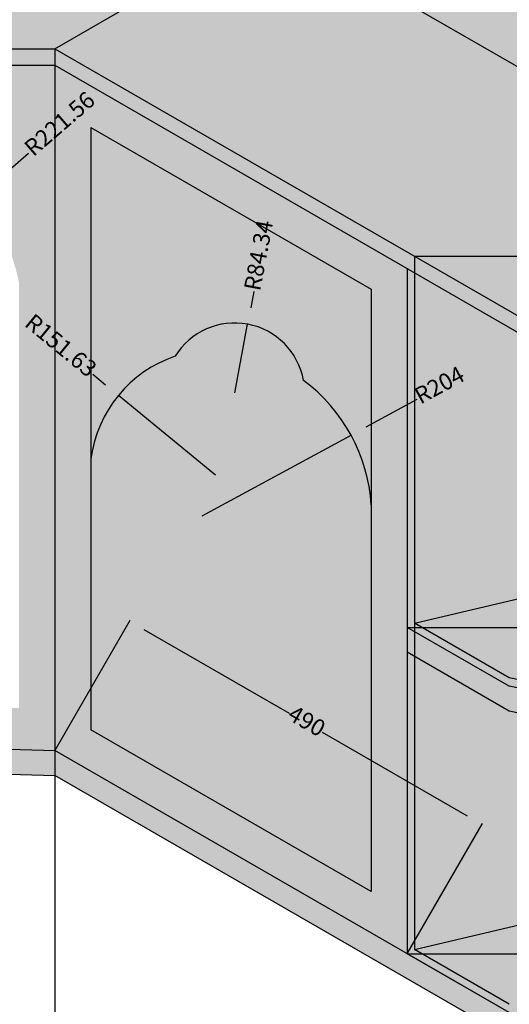
# Model space of a CAD drawing. Units: millimetres. Extents: x 78378 to 86415, y 148682 to 152721.
# Tile 10 of 18: x 80650 to 81240, y 149308 to 150495. Entities that reach past the tile are written whole.
import ezdxf

# ---------------------------------------------------------------- set-up
doc = ezdxf.new("R2010")
doc.units = ezdxf.units.MM
for name, color, linetype, lineweight in [('A-ANNO-DIMS', 2, 'Continuous', 18), ('A-FURN', 4, 'Continuous', 25), ('A-FURN-PATT', 32, 'Continuous', 13)]:
    doc.layers.add(name, color=color, linetype=linetype, lineweight=lineweight)
doc.styles.get("Standard").update_dxf_attribs({"font": 'arial.ttf'})
doc.dimstyles.new('ISO-25', dxfattribs={"dimtxt": 20, "dimasz": 20, "dimexe": 1.25, "dimexo": 0.625, "dimtad": 0, "dimdec": 1, "dimtxsty": 'Standard', "dimcen": 2.5, "dimadec": 0, "dimazin": 0, "dimtfac": 1, "dimtdec": 1, "dimtmove": 0, "dimatfit": 3, "dimfxl": 1, "dimarcsym": 0})

# ---------------------------------------------------------------- blocks, each defined once
blk = doc.blocks.new('*D27')
at = {"layer": 'A-ANNO-DIMS', "color": 0, "lineweight": -2, "transparency": 16777216}
for p, q in [((80692.9, 149614.5), (80783.2, 149771)), ((80799.9, 149759.9), (80974.8, 149658.9)), ((81189.7, 149534.9), (81014.8, 149635.8)), ((81117.3, 149369.5), (81207.6, 149526))]:
    blk.add_line(p, q, dxfattribs=at)
at = {"layer": 'A-ANNO-DIMS', "color": 0, "transparency": 16777216}
for points in [[(80801.6, 149762.8), (80798.3, 149757), (80782.6, 149769.9)], [(81191.3, 149537.8), (81188, 149532), (81207, 149524.9)]]:
    blk.add_solid(points, dxfattribs=at)
at = {"layer": 'Defpoints', "color": 0, "transparency": 16777216}
for p in [(80692.6, 149614), (81207, 149524.9), (81117, 149369)]:
    blk.add_point(p, dxfattribs=at)
at = {"layer": 'A-ANNO-DIMS', "color": 0, "transparency": 16777216, "insert": (80994.8, 149647.4), "char_height": 20, "attachment_point": 5, "rotation": 330}
blk.add_mtext('490', dxfattribs=at)
blk = doc.blocks.new('*D28')
at = {"layer": 'A-ANNO-DIMS', "color": 0, "lineweight": -2, "transparency": 16777216}
for p, q in [((81117.6, 149762.4), (81956.4, 149762.4)), ((81955.2, 149742.4), (81955.2, 149600)), ((81955.2, 149389), (81955.2, 149531.4)), ((81117.6, 149369), (81956.4, 149369))]:
    blk.add_line(p, q, dxfattribs=at)
at = {"layer": 'A-ANNO-DIMS', "color": 0, "transparency": 16777216}
for points in [[(81951.8, 149742.4), (81958.5, 149742.4), (81955.2, 149762.4)], [(81951.8, 149389), (81958.5, 149389), (81955.2, 149369)]]:
    blk.add_solid(points, dxfattribs=at)
at = {"layer": 'Defpoints', "color": 0, "transparency": 16777216}
for p in [(81117, 149762.4), (81955.2, 149762.4), (81117, 149369)]:
    blk.add_point(p, dxfattribs=at)
at = {"layer": 'A-ANNO-DIMS', "color": 0, "transparency": 16777216, "insert": (81955.2, 149565.7), "char_height": 20, "attachment_point": 5, "rotation": 90}
blk.add_mtext('393.4', dxfattribs=at)
blk = doc.blocks.new('*D29')
at = {"layer": 'A-ANNO-DIMS', "color": 0, "lineweight": -2, "transparency": 16777216}
for p, q in [((81126.3, 150210), (81956.4, 150210)), ((81955.2, 150190), (81955.2, 150021)), ((81955.2, 149782.4), (81955.2, 149951.4)), ((81117.6, 149762.4), (81956.4, 149762.4))]:
    blk.add_line(p, q, dxfattribs=at)
at = {"layer": 'A-ANNO-DIMS', "color": 0, "transparency": 16777216}
for points in [[(81951.8, 150190), (81958.5, 150190), (81955.2, 150210)], [(81951.8, 149782.4), (81958.5, 149782.4), (81955.2, 149762.4)]]:
    blk.add_solid(points, dxfattribs=at)
at = {"layer": 'Defpoints', "color": 0, "transparency": 16777216}
for p in [(81125.6, 150210), (81955.2, 150210), (81117, 149762.4)]:
    blk.add_point(p, dxfattribs=at)
at = {"layer": 'A-ANNO-DIMS', "color": 0, "transparency": 16777216, "insert": (81955.2, 149986.2), "char_height": 20, "attachment_point": 5, "rotation": 90}
blk.add_mtext('447.6', dxfattribs=at)
blk = doc.blocks.new('*D32')
at = {"layer": 'A-ANNO-DIMS', "color": 0, "lineweight": -2, "transparency": 16777216}
for p, q in [((80086.4, 150459.4), (80086.4, 148693.8)), ((80692.6, 150459.4), (80692.6, 148693.8)), ((80106.4, 148695), (80355.2, 148695)), ((80672.6, 148695), (80423.8, 148695))]:
    blk.add_line(p, q, dxfattribs=at)
at = {"layer": 'A-ANNO-DIMS', "color": 0, "transparency": 16777216}
for points in [[(80106.4, 148698.3), (80106.4, 148691.7), (80086.4, 148695)], [(80672.6, 148698.3), (80672.6, 148691.7), (80692.6, 148695)]]:
    blk.add_solid(points, dxfattribs=at)
at = {"layer": 'Defpoints', "color": 0, "transparency": 16777216}
for p in [(80086.4, 150460), (80692.6, 150460), (80692.6, 148695)]:
    blk.add_point(p, dxfattribs=at)
at = {"layer": 'A-ANNO-DIMS', "color": 0, "transparency": 16777216, "insert": (80389.5, 148695), "char_height": 20, "attachment_point": 5}
blk.add_mtext('606.2', dxfattribs=at)
blk = doc.blocks.new('*D64')
at = {"layer": 'A-ANNO-DIMS', "color": 0, "lineweight": -2, "transparency": 16777216}
for p, q in [((80660.8, 150333.8), (80614.5, 150293.7)), ((80431.9, 150135.6), (80599.4, 150280.6))]:
    blk.add_line(p, q, dxfattribs=at)
at = {"layer": 'A-ANNO-DIMS', "color": 0, "transparency": 16777216}
blk.add_solid([(80612.3, 150296.2), (80616.7, 150291.2), (80599.4, 150280.6)], dxfattribs=at)
at = {"layer": 'Defpoints', "color": 0, "transparency": 16777216}
for p in [(80599.4, 150280.6), (80431.9, 150135.6)]:
    blk.add_point(p, dxfattribs=at)
at = {"layer": 'A-ANNO-DIMS', "color": 0, "transparency": 16777216, "insert": (80699.9, 150367.7), "char_height": 20, "attachment_point": 5, "rotation": 40.8938}
blk.add_mtext('R221.56', dxfattribs=at)
blk = doc.blocks.new('*D66')
at = {"layer": 'A-ANNO-DIMS', "color": 0, "lineweight": -2, "transparency": 16777216}
for p, q in [((81128.6, 150037.1), (81067, 150003.6)), ((80870.1, 149896.7), (81049.4, 149994))]:
    blk.add_line(p, q, dxfattribs=at)
at = {"layer": 'A-ANNO-DIMS', "color": 0, "transparency": 16777216}
blk.add_solid([(81065.4, 150006.5), (81068.6, 150000.7), (81049.4, 149994)], dxfattribs=at)
at = {"layer": 'Defpoints', "color": 0, "transparency": 16777216}
for p in [(81049.4, 149994), (80870.1, 149896.7)]:
    blk.add_point(p, dxfattribs=at)
at = {"layer": 'A-ANNO-DIMS', "color": 0, "transparency": 16777216, "insert": (81157, 150052.4), "char_height": 20, "attachment_point": 5, "rotation": 28.4955}
blk.add_mtext('R204', dxfattribs=at)
blk = doc.blocks.new('*D67')
at = {"layer": 'A-ANNO-DIMS', "color": 0, "lineweight": -2, "transparency": 16777216}
for p, q in [((80738.3, 150067.6), (80753.7, 150054.9)), ((80886.2, 149945.8), (80769.1, 150042.1))]:
    blk.add_line(p, q, dxfattribs=at)
at = {"layer": 'A-ANNO-DIMS', "color": 0, "transparency": 16777216}
blk.add_solid([(80755.8, 150057.4), (80751.6, 150052.3), (80769.1, 150042.1)], dxfattribs=at)
at = {"layer": 'Defpoints', "color": 0, "transparency": 16777216}
for p in [(80769.1, 150042.1), (80886.2, 149945.8)]:
    blk.add_point(p, dxfattribs=at)
at = {"layer": 'A-ANNO-DIMS', "color": 0, "transparency": 16777216, "insert": (80698.3, 150100.4), "char_height": 20, "attachment_point": 5, "rotation": 320.5336}
blk.add_mtext('R151.63', dxfattribs=at)
blk = doc.blocks.new('*D68')
at = {"layer": 'A-ANNO-DIMS', "color": 0, "lineweight": -2, "transparency": 16777216}
for p, q in [((80932.2, 150167.2), (80928.5, 150147.6)), ((80909.2, 150045), (80924.8, 150127.9))]:
    blk.add_line(p, q, dxfattribs=at)
at = {"layer": 'A-ANNO-DIMS', "color": 0, "transparency": 16777216}
blk.add_solid([(80925.3, 150148.2), (80931.8, 150147), (80924.8, 150127.9)], dxfattribs=at)
at = {"layer": 'Defpoints', "color": 0, "transparency": 16777216}
for p in [(80924.8, 150127.9), (80909.2, 150045)]:
    blk.add_point(p, dxfattribs=at)
at = {"layer": 'A-ANNO-DIMS', "color": 0, "transparency": 16777216, "insert": (80940.4, 150210.4), "char_height": 20, "attachment_point": 5, "rotation": 79.3222}
blk.add_mtext('R84.34', dxfattribs=at)

msp = doc.modelspace()

# ---------------------------------------------------------------- hatches: boundary and pattern name
at = {"layer": 'A-FURN-PATT'}
h = msp.add_hatch(color=256, dxfattribs=at)
h.dxf.hatch_style = 1
h.paths.add_polyline_path([(78839.3276, 151040.0076), (78579.52, 151190.0076), (78579.52, 150470.0076), (78839.3276, 150320.0076)])
h.paths.add_polyline_path([(79073.1545, 150899.6469, 0.277779695), (79002.2645, 150996.3205, 0.791083931), (78917.9567, 150978.8719, 0.180448316), (78856.6481, 150853.0138), (78856.6481, 150350.6973), (79073.1545, 150484.318)])
h.paths.add_polyline_path([(79073.1545, 151175.0076), (78856.6481, 151050.0076), (78856.6481, 150853.0138, -0.180448316), (78917.9567, 150978.8719, -0.791083931), (79002.2645, 150996.3205, -0.277779695), (79073.1545, 150899.6469)])
h.paths.add_polyline_path([(79341.6224, 151350.0076), (79099.1352, 151490.0076), (78596.8405, 151200.0076), (78839.3276, 151060.0076)])
h.paths.add_polyline_path([(79904.5389, 151675.0076), (79662.0518, 151815.0076), (79099.1352, 151490.0076), (79341.6224, 151350.0076)])
h.paths.add_polyline_path([(80389.5131, 151955.0076), (80389.5131, 152235.0076), (79662.0518, 151815.0076), (79904.5389, 151675.0076)])
h.paths.add_polyline_path([(80389.5131, 151955.0076), (80164.3465, 151825.0076), (80164.3465, 151105.0076), (80614.6797, 151105.0076), (80614.6797, 151825.0076)])
edge = h.paths.add_edge_path(flags=16)
edge.add_spline(control_points=[(80216.308, 151728.251), (80227.1854, 151732.981), (80256.3301, 151745.6544), (80298.41, 151761.9595), (80340.2597, 151805.855), (80391.0771, 151782.0404), (80454.0396, 151805.7581), (80496.5007, 151742.4095), (80543.8218, 151733.4043), (80562.7182, 151729.8083)], knot_values=[0, 0, 0, 0, 35.543746761, 95.235753469, 136.367675126, 200.932981967, 236.726410811, 322.889934976, 380.170273667, 380.170273667, 380.170273667, 380.170273667], degree=3, periodic=0)
edge.add_line((80562.7182, 151729.8083), (80562.7182, 151165.0076))
edge.add_line((80562.7182, 151165.0076), (80216.308, 151165.0076))
edge.add_line((80216.308, 151165.0076), (80216.308, 151728.251))
h.paths.add_polyline_path([(80632.0002, 152095.0076), (80389.5131, 152235.0076), (80389.5131, 151955.0076), (80614.6797, 151825.0076), (80632.0002, 151815.0076)])
h.paths.add_polyline_path([(80867.7794, 151958.8805), (80632.0002, 152095.0076), (80632.0002, 151815.0076), (80632.0002, 151510.0076), (80867.7794, 151373.8805)])
h.paths.add_polyline_path([(80147.026, 151495.8203, 0.18918979), (80063.5671, 151597.7244, 0.788261355), (79979.2691, 151580.5832, 0.160726132), (79904.5389, 151413.5769), (79904.5389, 150955.0076), (80147.026, 151095.0076)])
h.paths.add_polyline_path([(80147.026, 151815.0076), (79904.5389, 151675.0076), (79904.5389, 151413.5769, -0.160726132), (79979.2691, 151580.5832, -0.788261355), (80063.5671, 151597.7244, -0.18918979), (80147.026, 151495.8203)])
h.paths.add_polyline_path([(79887.2184, 151645.0076), (79640.4011, 151502.5076), (79640.4011, 151262.3325, -0.160726132), (79715.1313, 151429.3387, -0.788261355), (79799.4294, 151446.48, -0.21290578), (79887.2184, 151328.7247)])
h.paths.add_polyline_path([(79799.4294, 151446.48, 0.788261355), (79715.1313, 151429.3387, 0.160726132), (79640.4011, 151262.3325), (79640.4011, 150822.5076), (79887.2184, 150965.0076), (79887.2184, 151328.7247, 0.21290578)])
h.paths.add_polyline_path([(79605.7601, 151482.5076), (79358.9429, 151340.0076), (79358.9429, 151100.0701, -0.160726132), (79433.6731, 151267.0764, -0.788261355), (79517.9711, 151284.2176, -0.21290578), (79605.7601, 151166.4623)])
h.paths.add_polyline_path([(79605.7601, 151166.4623, 0.21290578), (79517.9711, 151284.2176, 0.788261355), (79433.6731, 151267.0764, 0.160726132), (79358.9429, 151100.0701), (79358.9429, 150742.9831), (79419.0877, 150694.7323), (79605.7601, 150802.5076)])
edge = h.paths.add_edge_path(flags=0)
edge.add_spline(control_points=[(81152.4356, 151098.7676), (81105.7208, 151145.9466), (81038.6136, 151213.7208), (80882.3866, 151214.1938), (80797.4434, 151311.2997), (80711.8686, 151340.3754), (80681.7691, 151350.6023)], knot_values=[0, 0, 0, 0, 188.233441, 270.4032752, 445.451792012, 540.428588287, 540.428588287, 540.428588287, 540.428588287], degree=3, periodic=0)
edge.add_line((80683.4538, 151350.0269), (80683.4538, 151104.8792))
edge.add_line((80683.4538, 151104.8792), (81152.4356, 150851.399))
edge.add_line((81152.4356, 150851.399), (81152.4356, 151098.7676))
edge = h.paths.add_edge_path(flags=0)
edge.add_spline(control_points=[(80912.9018, 151027.1103), (80892.3742, 151034.1027), (80860.1663, 151045.0739), (80835.5097, 151068.1214), (80826.5679, 151076.4797)], knot_values=[0, 0, 0, 0, 63.98405104, 100.391424282, 100.391424282, 100.391424282, 100.391424282], degree=3, periodic=0)
edge.add_arc((80830.0414, 151081.2992), 5.9407, 100.9277276, 234.2187381, ccw=False)
edge.add_spline(control_points=[(80828.9152, 151087.1322), (80837.857, 151078.7739), (80862.5136, 151055.7263), (80894.7215, 151044.7552), (80915.2491, 151037.7628)], knot_values=[0, 0, 0, 0, 36.407373242, 100.391424282, 100.391424282, 100.391424282, 100.391424282], degree=3, periodic=0)
edge.add_arc((80914.7882, 151032.2795), 5.5026, -107.9540399, 85.195579, ccw=False)
h.paths.add_polyline_path([(81238.218, 151110.0076), (80632.0002, 151460.0076), (80632.0002, 151105.0076), (81238.218, 150755.0076)])
edge = h.paths.add_edge_path(flags=16)
edge.add_line((81152.4356, 150851.399), (80683.4538, 151104.8792))
edge.add_line((80683.4538, 151104.8792), (80683.4538, 151350.0279))
edge.add_spline(control_points=[(80681.7691, 151350.6023), (80711.8686, 151340.3754), (80797.4434, 151311.2997), (80882.3866, 151214.1938), (81038.6136, 151213.7208), (81105.7208, 151145.9466), (81152.4356, 151098.7676)], knot_values=[0, 0, 0, 0, 94.976796275, 270.025313088, 352.195147288, 540.428588287, 540.428588287, 540.428588287, 540.428588287], degree=3, periodic=0)
edge.add_line((81152.4356, 151098.7676), (81152.4356, 150851.399))
edge = h.paths.add_edge_path(flags=0)
edge.add_spline(control_points=[(80912.9018, 151027.1103), (80892.3742, 151034.1027), (80860.1663, 151045.0739), (80835.5097, 151068.1214), (80826.5679, 151076.4797)], knot_values=[0, 0, 0, 0, 63.98405104, 100.391424282, 100.391424282, 100.391424282, 100.391424282], degree=3, periodic=0)
edge.add_arc((80830.0414, 151081.2992), 5.9407, 100.9277276, 234.2187381, ccw=False)
edge.add_spline(control_points=[(80828.9152, 151087.1322), (80837.857, 151078.7739), (80862.5136, 151055.7263), (80894.7215, 151044.7552), (80915.2491, 151037.7628)], knot_values=[0, 0, 0, 0, 36.407373242, 100.391424282, 100.391424282, 100.391424282, 100.391424282], degree=3, periodic=0)
edge.add_arc((80914.7882, 151032.2795), 5.5026, -107.7417882, 85.195579, ccw=False)
h.paths.add_polyline_path([(81498.0256, 151255.0076), (81238.218, 151110.0076), (81238.218, 150755.0076), (81498.0256, 150905.0076)])
edge = h.paths.add_edge_path(flags=16)
edge.add_spline(control_points=[(81152.4356, 151098.7676), (81105.7208, 151145.9466), (81038.6136, 151213.7208), (80882.3866, 151214.1938), (80797.4434, 151311.2997), (80711.8686, 151340.3754), (80681.7691, 151350.6023)], knot_values=[0, 0, 0, 0, 188.233441, 270.4032752, 445.451792012, 540.428588287, 540.428588287, 540.428588287, 540.428588287], degree=3, periodic=0)
edge.add_line((80683.4538, 151350.0279), (80683.4538, 151104.8792))
edge.add_line((80683.4538, 151104.8792), (81152.4356, 150851.399))
edge.add_line((81152.4356, 150851.399), (81152.4356, 151098.7676))
h.paths.add_polyline_path([(81453.9904, 151280.4314), (80867.7794, 151618.8805), (80867.7794, 151373.8805), (81238.218, 151160.0076)])
edge = h.paths.add_edge_path(flags=16)
edge.add_line((81189.2304, 151297.6373), (81114.4166, 151300.2154))
edge.add_arc((81412.0967, 151394.0167), 312.1092, 179.7569303, 197.4900342, ccw=False)
edge.add_ellipse((81154.0183, 151392.0436), major_axis=(-54.0264, 3.6301), ratio=0.221796934, start_angle=0, end_angle=0.3517985, ccw=False)
edge.add_ellipse((81154.0183, 151392.0436), major_axis=(-54.0264, 3.6301), ratio=0.221796934, start_angle=180, end_angle=360, ccw=False)
edge.add_spline(control_points=[(81196.1844, 151321.9476), (81224.9802, 151347.1455), (81266.8846, 151383.8144), (81222.0354, 151387.0304), (81208.0056, 151388.0364)], knot_values=[0, 0, 0, 0, 75.091751734, 109.275804387, 109.275804387, 109.275804387, 109.275804387], degree=3, periodic=0)
edge.add_arc((80751.9112, 151435.6145), 458.5693, 342.4891602, 345.646172, ccw=False)
edge = h.paths.add_edge_path(flags=0)
edge.add_spline(control_points=[(81196.6193, 151323.657), (81197.893, 151324.7717), (81199.1654, 151325.8858), (81209.0233, 151334.5343), (81217.3959, 151341.9835), (81228.0928, 151352.5012), (81231.3883, 151355.9524), (81236.9493, 151362.4395), (81239.214, 151365.4773), (81241.4987, 151369.416), (81242.064, 151370.5542), (81242.9187, 151372.6971), (81243.2076, 151373.7015), (81243.5012, 151375.5539), (81243.5065, 151376.4), (81243.2432, 151377.9407), (81242.9775, 151378.6373), (81242.1402, 151379.937), (81241.5659, 151380.5416), (81240.2039, 151381.533), (81239.4963, 151381.9384), (81237.0619, 151383.0663), (81235.0242, 151383.6999), (81230.352, 151384.7569), (81227.7173, 151385.1826), (81221.9118, 151385.9145), (81218.7193, 151386.2133), (81213.7912, 151386.6115), (81212.1252, 151386.7359), (81209.6196, 151386.9181), (81208.7865, 151386.9779), (81207.9009, 151387.0432)], knot_values=[0.015487437, 0.015487437, 0.015487437, 0.015487437, 3.337879569, 3.337879569, 25.851306242, 25.851306242, 37.52811308, 37.52811308, 49.204919918, 49.204919918, 54.285093801, 54.285093801, 59.365267683, 59.365267683, 64.445441566, 64.445441566, 69.525615449, 69.525615449, 74.605789331, 74.605789331, 78.493667847, 78.493667847, 86.255670953, 86.255670953, 94.017674059, 94.017674059, 102.202265559, 102.202265559, 106.294561309, 106.294561309, 108.325221747, 108.325221747, 108.325221747, 108.325221747], degree=3, periodic=0)
edge = h.paths.add_edge_path(flags=16)
edge.add_arc((81034.1732, 151350.4693), 42.5822, 231.2679035, 306.151846, ccw=False)
edge.add_line((81007.5303, 151317.2517), (81007.5303, 151395.181))
edge.add_ellipse((81033.412, 151394.7791), major_axis=(-25.8816, 0.4538), ratio=0.23894509, start_angle=0, end_angle=0.1147075, ccw=False)
edge.add_ellipse((81033.412, 151394.7791), major_axis=(-25.8816, 0.4538), ratio=0.23894509, start_angle=181.1677709, end_angle=358.9476457, ccw=False)
edge.add_ellipse((81033.412, 151395.7791), major_axis=(-25.8816, 0.4538), ratio=0.23894509, start_angle=180, end_angle=360.1147075, ccw=False)
edge.add_ellipse((81033.412, 151395.7791), major_axis=(-25.8816, 0.4538), ratio=0.23894509, start_angle=178.9476457, end_angle=180, ccw=False)
edge.add_line((81059.2936, 151395.1778), (81059.2936, 151394.3772))
edge.add_ellipse((81033.412, 151394.7791), major_axis=(-25.8816, 0.4538), ratio=0.23894509, start_angle=180, end_angle=180.1147075, ccw=False)
edge.add_ellipse((81033.412, 151394.7791), major_axis=(-25.8816, 0.4538), ratio=0.23894509, start_angle=3.6903098, end_angle=176.4406503, ccw=False)
edge.add_line((81059.2936, 151393.3388), (81059.2936, 151316.086))
h.paths.add_polyline_path([(80951.9355, 151343.9568), (80909.6838, 151362.4635), (80904.0219, 151443.9615, -0.381333076), (80987.2169, 151411.3717)], flags=16)
h = msp.add_hatch(color=256, dxfattribs=at)
h.dxf.hatch_style = 1
h.paths.add_polyline_path([(80389.8136, 150935.1811), (80389.5131, 151105.0076), (80164.3465, 151105.0076), (79904.5389, 150955.0076), (79433.5848, 150683.1022), (79459.4128, 150662.3818), (79243.9048, 150537.9582), (79160.4069, 150518.1674), (78839.3276, 150320.0076), (78579.52, 150470.0076), (78570.8597, 150475.0076), (78570.8597, 150465.0076), (78570.8597, 149885.0076)])
h.paths.add_polyline_path([(80086.4042, 150460.0076), (79826.5966, 150610.0076), (78570.8597, 149885.0076), (78830.6674, 149735.0076)])
h.paths.add_polyline_path([(79540.8001, 150161.0557), (79217.3967, 149974.3386), (78980.9166, 150110.8705), (79304.32, 150297.5875)], flags=16)
h.paths.add_polyline_path([(79506.159, 150161.0557), (79217.3967, 149994.3386), (79015.5576, 150110.8705), (79304.32, 150277.5875)], flags=0)
edge = h.paths.add_edge_path(flags=0)
edge.add_arc((79247.8636, 150177.1541), 137.9799, 256.0025928, 293.5594109)
edge.add_arc((79240.7671, 150078.2605), 68.0855, 336.099104, 387.3696877)
edge.add_ellipse((79258.3074, 150109.4852), major_axis=(-42.6234, -1.6591), ratio=0.160428429, start_angle=0, end_angle=179.0977279, ccw=False)
edge.add_arc((79285.2112, 150074.2509), 77.2096, 155.1233104, 203.6557939)
edge = h.paths.add_edge_path(flags=0)
edge.add_ellipse((79258.6958, 150110.8297), major_axis=(-42.6234, -1.6591), ratio=0.160428429, start_angle=350.6039412, end_angle=356.2289762)
edge.add_line((79219.169, 150111.8937), (79218.3268, 150109.4141))
edge.add_arc((79262.4675, 150032.9602), 88.2813, 112.3931229, 120, ccw=False)
h.paths.add_polyline_path([(79287.0625, 150086.9703, -0.247702064), (79288.1967, 150077.2955, -0.390476513), (79265.4731, 150072.5438, -0.487261526), (79264.079, 150082.3769, 0.395604326)], flags=0)
h.paths.add_polyline_path([(80389.5131, 150935.0076), (79826.5966, 150610.0076), (80086.4042, 150460.0076), (80692.622, 150460.0076), (80952.4296, 150610.0076)])
edge = h.paths.add_edge_path(flags=16)
edge.add_ellipse((80392.4466, 150825.601), major_axis=(-133.0757, 7.722), ratio=0.42449957, start_angle=0, end_angle=360)
edge = h.paths.add_edge_path(flags=0)
edge.add_spline(control_points=[(80269.3541, 150832.7436), (80269.2919, 150831.672), (80269.3503, 150830.5922), (80269.7341, 150828.3361), (80270.0612, 150827.1587), (80271.0461, 150824.6748), (80271.7052, 150823.3692), (80273.4061, 150820.6503), (80274.4481, 150819.2381), (80276.9366, 150816.3509), (80278.3828, 150814.8762), (80282.5858, 150811.0913), (80285.6261, 150808.7701), (80292.6031, 150804.2267), (80296.5388, 150802.0041), (80305.195, 150797.7581), (80309.9151, 150795.7344), (80320.0112, 150791.96), (80325.387, 150790.2092), (80339.2162, 150786.315), (80347.9578, 150784.3563), (80366.0679, 150781.2568), (80375.4359, 150780.1158), (80394.3093, 150778.7158), (80403.8142, 150778.4568), (80422.4656, 150778.8319), (80431.6115, 150779.4662), (80449.0608, 150781.5838), (80457.3636, 150783.0675), (80472.6699, 150786.7766), (80479.6726, 150789.0033), (80490.1894, 150793.2813), (80494.1268, 150795.1967), (80501.0146, 150799.1885), (80503.9632, 150801.2651), (80508.2066, 150804.9015), (80509.73, 150806.4609), (80512.1996, 150809.4942), (80513.1456, 150810.9657), (80514.4291, 150813.5431), (80514.8436, 150814.6688), (80515.3984, 150816.8625), (80515.5405, 150817.9315), (80515.5801, 150820.098), (80515.4773, 150821.1978), (80514.9905, 150823.5062), (80514.6047, 150824.7154), (80513.4854, 150827.2641), (80512.7511, 150828.6027), (80510.8872, 150831.3809), (80509.7578, 150832.8196), (80507.0873, 150835.7513), (80505.5466, 150837.2439), (80501.0624, 150841.0944), (80497.8199, 150843.4576), (80490.4174, 150848.062), (80486.2582, 150850.3037), (80477.1448, 150854.5643), (80472.1909, 150856.5835), (80461.6275, 150860.3245), (80456.0182, 150862.0465), (80441.7332, 150865.8127), (80432.7885, 150867.6675), (80414.3391, 150870.5317), (80404.8349, 150871.5411), (80385.7707, 150872.6572), (80376.2113, 150872.764), (80357.5444, 150872.0728), (80348.4375, 150871.2748), (80331.1682, 150868.83), (80323.0064, 150867.1827), (80309.472, 150863.5363), (80303.8628, 150861.6593), (80293.8018, 150857.5401), (80289.3512, 150855.2969), (80282.7757, 150851.2345), (80280.3473, 150849.4579), (80276.2606, 150845.9127), (80274.604, 150844.1458), (80272.3157, 150841.1243), (80271.5358, 150839.8454), (80270.3496, 150837.3879), (80269.9417, 150836.2101), (80269.5065, 150834.2815), (80269.3988, 150833.5143), (80269.3541, 150832.7436)], knot_values=[0, 0, 0, 0, 0.09750046, 0.09750046, 0.19500092, 0.19500092, 0.292501379, 0.292501379, 0.390001839, 0.390001839, 0.487502299, 0.487502299, 0.638803224, 0.638803224, 0.790104149, 0.790104149, 0.941405074, 0.941405074, 1.092705999, 1.092705999, 1.312817101, 1.312817101, 1.532928203, 1.532928203, 1.753039304, 1.753039304, 1.973150406, 1.973150406, 2.193261508, 2.193261508, 2.413372609, 2.413372609, 2.569860633, 2.569860633, 2.726348657, 2.726348657, 2.844186582, 2.844186582, 2.962024507, 2.962024507, 3.060233876, 3.060233876, 3.158443245, 3.158443245, 3.256652615, 3.256652615, 3.354861984, 3.354861984, 3.453071354, 3.453071354, 3.551280723, 3.551280723, 3.649490093, 3.649490093, 3.80392773, 3.80392773, 3.958365368, 3.958365368, 4.112803006, 4.112803006, 4.267240644, 4.267240644, 4.489203495, 4.489203495, 4.711166346, 4.711166346, 4.933129197, 4.933129197, 5.155092048, 5.155092048, 5.3770549, 5.3770549, 5.557853609, 5.557853609, 5.738652318, 5.738652318, 5.872395556, 5.872395556, 6.006138794, 6.006138794, 6.109604996, 6.109604996, 6.213071198, 6.213071198, 6.283185307, 6.283185307, 6.283185307, 6.283185307], degree=3, periodic=0)
edge = h.paths.add_edge_path(flags=0)
edge.add_ellipse((80392.4466, 150825.601), major_axis=(-101.8398, 3.3923), ratio=0.403492477, start_angle=0, end_angle=360)
edge = h.paths.add_edge_path(flags=0)
edge.add_ellipse((80391.1657, 150858.3746), major_axis=(9.0882, -0.6733), ratio=0.351354129, start_angle=0, end_angle=360)
h.paths.add_polyline_path([(80952.4296, 150610.0076), (80692.622, 150460.0076), (81361.2342, 150073.9842), (81649.9628, 150052.7286), (81766.4935, 150120.0076), (81766.4935, 150140.0076), (81564.9025, 150256.3963), (81564.8884, 150096.1963), (81538.9076, 150111.1963), (81538.9217, 150271.3963)])
h.paths.add_polyline_path([(81539.0357, 151571.3305), (80867.7794, 151958.8805), (80867.7794, 151618.8805), (81498.0256, 151255.0076), (81498.0256, 150905.0076), (81238.218, 150755.0076), (81538.9488, 150581.3806)])
h.paths.add_polyline_path([(81766.4935, 151440.0076), (81565.0164, 151556.3305), (81564.9296, 150566.3806), (81766.4935, 150450.0076)])
edge = h.paths.add_edge_path()
edge.add_line((81564.9296, 150566.3806), (81564.9137, 150384.6289))
edge.add_ellipse((81552.1304, 150358.5718), major_axis=(52.6272, 3.506), ratio=0.495899055, start_angle=367.5169757, end_angle=420.0564686, ccw=False)
edge.add_ellipse((81552.1304, 150358.5718), major_axis=(52.6272, 3.506), ratio=0.495899055, start_angle=351.729742, end_angle=367.5169757, ccw=False)
edge.add_ellipse((81552.1304, 150345.5016), major_axis=(52.6272, 3.506), ratio=0.495899055, start_angle=352.5116949, end_angle=366.3006092, ccw=False)
edge.add_line((81603.4463, 150342.2039), (81603.5064, 150340.4475))
edge.add_ellipse((81552.1304, 150332.128), major_axis=(52.6272, 3.506), ratio=0.495899055, start_angle=353.6729654, end_angle=365.3867997, ccw=False)
edge.add_ellipse((81552.1304, 150332.128), major_axis=(52.6272, 3.506), ratio=0.495899055, start_angle=350.9388331, end_angle=353.6729654)
edge.add_line((81603.8688, 150329.855), (81604.0442, 150324.7302))
edge.add_ellipse((81552.1304, 150317.7418), major_axis=(52.6272, 3.506), ratio=0.495899055, start_angle=355.2176746, end_angle=363.8553364, ccw=False)
edge.add_ellipse((81552.1304, 150317.7418), major_axis=(52.6272, 3.506), ratio=0.495899055, start_angle=341.3250873, end_angle=355.2176746, ccw=False)
edge.add_ellipse((81552.1304, 150317.7418), major_axis=(52.6272, 3.506), ratio=0.495899055, start_angle=293.4661701, end_angle=341.3250873, ccw=False)
edge.add_line((81564.9057, 150292.9664), (81564.9025, 150256.3963))
edge.add_line((81564.9025, 150256.3963), (81766.4935, 150140.0076))
edge.add_line((81766.4935, 150140.0076), (81766.4935, 150450.0076))
edge.add_line((81766.4935, 150450.0076), (81564.9296, 150566.3806))
h.paths.add_polyline_path([(81525.5713, 150321.598), (81526.5985, 150321.3069), (81528.6771, 150320.947)])
h.paths.add_polyline_path([(81512.7903, 150326.1129), (81514.5058, 150325.3887), (81512.538, 150326.2678)])
h.paths.add_polyline_path([(81533.2148, 150320.1615), (81534.6952, 150319.9052), (81536.5995, 150319.7557)])
h.paths.add_polyline_path([(81518.622, 150323.6513), (81519.227, 150323.3959), (81521.289, 150322.8116)])
h.paths.add_polyline_path([(81501.2183, 150336.2599), (81500.3543, 150338.1339), (81499.7815, 150340.0494), (81499.5032, 150341.9955), (81499.5032, 150343.7257), (81499.7584, 150345.5905), (81500.2766, 150347.4549), (81501.0551, 150349.3095), (81501.0967, 150349.3937), (81501.1389, 150349.4778), (81500.9978, 150349.7496), (81500.8628, 150350.0225), (81499.5032, 150355.0658), (81499.9591, 150359.5002), (81501.8982, 150363.9083), (81505.2653, 150368.1646), (81509.9647, 150372.1482), (81515.8627, 150375.7459), (81522.7918, 150378.8553), (81530.555, 150381.3882), (81538.9315, 150383.2724), (81538.9488, 150581.3806), (80632.0002, 151105.0076), (80389.5131, 151105.0076), (80389.8142, 150934.8338), (80952.4296, 150610.0076), (81538.9217, 150271.3963), (81538.9234, 150291.7194), (81538.8752, 150291.721), (81530.1915, 150292.8239), (81522.1802, 150294.6904), (81515.0866, 150297.2633), (81509.8635, 150299.9959), (81505.6084, 150303.1351), (81502.419, 150306.6088), (81500.3683, 150310.3375), (81499.5032, 150314.2358), (81499.5032, 150315.9659), (81499.8206, 150318.1159), (81500.487, 150320.2634), (81501.4979, 150322.3941), (81500.487, 150324.4233), (81499.8206, 150326.5039), (81499.5032, 150328.622), (81499.5032, 150330.3521), (81499.7815, 150332.3262), (81500.3543, 150334.2992)])
h = msp.add_hatch(color=256, dxfattribs=at)
h.dxf.hatch_style = 1
h.paths.add_polyline_path([(79090.475, 151205.0076), (78839.3276, 151060.0076), (78839.3276, 150320.0076), (79090.475, 150475.0076)])
h.paths.add_polyline_path([(79073.1545, 151175.0076), (79073.1545, 150899.6469, -0.04544363), (79073.1545, 150878.5653), (79073.1545, 150484.318), (78856.6481, 150350.6973), (78856.6481, 150814.5249, -0.048157161), (78856.6481, 150853.0138), (78856.6481, 151050.0076)], flags=16)
h.paths.add_polyline_path([(79358.9429, 151340.0076), (79605.7601, 151482.5076), (79605.7601, 150802.5076), (79419.0877, 150694.7323), (79433.5848, 150683.1022), (79623.0806, 150792.5076), (79623.0806, 151512.5076), (79341.6224, 151350.0076), (79341.6224, 150756.8784), (79358.9429, 150742.9831)])
h.paths.add_polyline_path([(79341.6224, 151350.0076), (79090.475, 151205.0076), (79090.475, 150475.0076), (79160.4069, 150518.1674), (79107.7955, 150505.6973), (79107.7955, 151195.0076), (79109.5275, 151196.0076), (79324.3018, 151320.0076), (79324.3018, 150770.7736), (79341.6224, 150756.8784)])
h.paths.add_polyline_path([(79887.2184, 151645.0076), (79887.2184, 151665.0076), (79623.0806, 151512.5076), (79623.0806, 150792.5076), (79887.2184, 150945.0076), (79887.2184, 150965.0076), (79640.4011, 150822.5076), (79640.4011, 151502.5076)])
h.paths.add_polyline_path([(79904.5389, 151655.0076), (79887.2184, 151645.0076), (79887.2184, 150965.0076), (79904.5389, 150975.0076)])
h.paths.add_polyline_path([(80164.3465, 151825.0076), (80147.026, 151815.0076), (80147.026, 151095.0076), (80164.3465, 151105.0076)])
h.paths.add_polyline_path([(80632.0002, 151510.0076), (80632.0002, 151490.0076), (81238.218, 151140.0076), (81471.6045, 151270.2619), (81453.9904, 151280.4314), (81238.218, 151160.0076)])
h.paths.add_polyline_path([(80632.0002, 151490.0076), (80632.0002, 151470.0076), (81238.218, 151120.0076), (81489.2186, 151260.0924), (81471.6045, 151270.2619), (81238.218, 151140.0076)])
h.paths.add_polyline_path([(80632.0002, 151460.0076), (80632.0002, 151105.0076), (81238.218, 150755.0076), (81238.218, 151110.0076)])
edge = h.paths.add_edge_path(flags=16)
edge.add_spline(control_points=[(80681.7691, 151350.6023), (80711.8686, 151340.3754), (80797.4434, 151311.2997), (80882.3866, 151214.1938), (81038.6136, 151213.7208), (81105.7208, 151145.9466), (81152.4356, 151098.7676)], knot_values=[0, 0, 0, 0, 94.976796275, 270.025313088, 352.195147288, 540.428588287, 540.428588287, 540.428588287, 540.428588287], degree=3, periodic=0)
edge.add_line((81152.4356, 151098.7676), (81152.4356, 150851.399))
edge.add_line((81152.4356, 150851.399), (80683.4538, 151104.8792))
edge.add_line((80683.4538, 151104.8792), (80683.4538, 151350.027))
edge = h.paths.add_edge_path(flags=0)
edge.add_spline(control_points=[(80828.9152, 151087.1322), (80837.857, 151078.7739), (80862.5136, 151055.7263), (80894.7215, 151044.7552), (80915.2491, 151037.7628)], knot_values=[0, 0, 0, 0, 36.407373242, 100.391424282, 100.391424282, 100.391424282, 100.391424282], degree=3, periodic=0)
edge.add_arc((80914.7882, 151032.2795), 5.5026, -107.9540399, 85.195579, ccw=False)
edge.add_spline(control_points=[(80912.9018, 151027.1103), (80892.3742, 151034.1027), (80860.1663, 151045.0739), (80835.5097, 151068.1214), (80826.5679, 151076.4797)], knot_values=[0, 0, 0, 0, 63.98405104, 100.391424282, 100.391424282, 100.391424282, 100.391424282], degree=3, periodic=0)
edge.add_arc((80830.0414, 151081.2992), 5.9407, 100.9277276, 234.2187381, ccw=False)
h.paths.add_polyline_path([(80632.0002, 151815.0076), (80614.6797, 151825.0076), (80614.6797, 151105.0076), (80632.0002, 151105.0076)])
h.paths.add_polyline_path([(81498.0256, 151255.0076), (81489.2186, 151260.0924), (81238.218, 151120.0076), (80632.0002, 151470.0076), (80632.0002, 151460.0076), (81238.218, 151110.0076)])
h.paths.add_polyline_path([(78596.8405, 151200.0076), (78579.52, 151190.0076), (78839.3276, 151040.0076), (78839.3276, 151060.0076)])
h.paths.add_polyline_path([(78596.8405, 151200.0076), (78579.52, 151210.0076), (78579.52, 151190.0076)])
h.paths.add_polyline_path([(78579.52, 151210.0076), (78570.8597, 151205.0076), (78570.8597, 150475.0076), (78579.52, 150470.0076)])
h = msp.add_hatch(color=256, dxfattribs=at)
h.dxf.hatch_style = 1
h.paths.add_polyline_path([(80692.622, 150460.0076), (80086.4042, 150460.0076), (80086.4042, 150440.0076), (80692.622, 150440.0076)])
h = msp.add_hatch(color=256, dxfattribs=at)
h.dxf.hatch_style = 1
h.paths.add_polyline_path([(80692.622, 150460.0076), (80692.622, 150440.0076), (81125.6347, 150190.0076), (81125.6347, 150210.0076)])
h = msp.add_hatch(color=256, dxfattribs=at)
h.dxf.hatch_style = 1
h.paths.add_polyline_path([(80692.622, 150440.0076), (80086.4042, 150440.0076), (80086.4042, 149630.0076), (80692.622, 149614.0076)])
h.paths.add_polyline_path([(80293.421, 150335.1041, -0.693913747), (80505.0284, 150344.716, -0.266337997), (80649.3207, 150178.1039), (80649.3207, 149665.1505), (80129.7055, 149678.8648), (80129.7055, 150178.1039, -0.257326206)], flags=16)
h.paths.add_polyline_path([(80060.4234, 150384.3024), (79809.2761, 150239.3024), (79809.2761, 150141.6366), (80060.4234, 150286.6366)])
h.paths.add_polyline_path([(80086.4042, 150399.3024), (80086.4042, 150440.0076), (79783.2953, 150265.0076), (79783.2953, 150224.3024)])
edge = h.paths.add_edge_path(flags=16)
edge.add_arc((79946.6302, 150348.8763), 10.7636, -18.3817969, 28.0331994, ccw=False)
edge.add_spline(control_points=[(79956.8447, 150345.482), (79949.4862, 150336.2391), (79933.8528, 150316.6023), (79908.9507, 150312.562), (79895.7699, 150310.4234)], knot_values=[0, 0, 0, 0, 34.225683992, 72.713576575, 72.713576575, 72.713576575, 72.713576575], degree=3, periodic=0)
edge.add_arc((79899.3869, 150314.0155), 5.0977, 123.6496153, 224.8024751, ccw=False)
edge.add_spline(control_points=[(79896.5622, 150318.259), (79909.861, 150320.2803), (79934.7821, 150324.0679), (79949.3412, 150344.4361), (79956.131, 150353.935)], knot_values=[0, 0, 0, 0, 38.487892583, 72.123319114, 72.123319114, 72.123319114, 72.123319114], degree=3, periodic=0)
h.paths.add_polyline_path([(80086.4042, 150399.3024), (80060.4234, 150384.3024), (80060.4234, 150286.6366), (80086.4042, 150301.6366)], flags=17)
h.paths.add_polyline_path([(79809.2761, 150239.3024), (79783.2953, 150224.3024), (79783.2953, 150126.6366), (79809.2761, 150141.6366)])
h = msp.add_hatch(color=256, dxfattribs=at)
h.dxf.hatch_style = 1
h.paths.add_polyline_path([(81116.9744, 150195.0076), (80692.622, 150440.0076), (80692.622, 149614.0076), (81116.9744, 149369.0076)])
h.paths.add_polyline_path([(80735.9233, 150365.0076), (81073.6732, 150170.0076), (81073.6732, 149444.0076), (80735.9233, 149639.0076)], flags=16)
h = msp.add_hatch(color=256, dxfattribs=at)
h.dxf.hatch_style = 1
h.paths.add_polyline_path([(81239.9694, 149691.4023), (81125.6347, 149757.4135), (81125.6347, 149727.4135), (81239.9694, 149661.4023), (81645.2499, 149577.4135), (81670.0493, 149591.7314), (81766.4935, 149647.4135), (81766.4935, 149657.4135), (81749.173, 149667.4135), (81645.2499, 149607.4135)])
h.paths.add_polyline_path([(81239.9694, 149701.4023), (81125.6347, 149767.4135), (81125.6347, 149757.4135), (81239.9694, 149691.4023), (81645.2499, 149607.4135), (81749.173, 149667.4135), (81740.5127, 149672.4135), (81645.2499, 149617.4135)])
h.paths.add_polyline_path([(81116.9744, 150195.0076), (80692.622, 150440.0076), (80692.622, 149614.0076), (81116.9744, 149369.0076)])
h.paths.add_polyline_path([(81073.6732, 149444.0076), (80735.9233, 149639.0076), (80735.9233, 150365.0076), (81073.6732, 150170.0076)], flags=16)
h.paths.add_polyline_path([(81125.6347, 149727.4135), (81116.9744, 149732.4135), (81116.9744, 149369.0076), (81239.9694, 149297.9965), (81239.9694, 149307.9965), (81125.6347, 149374.0076)])
h.paths.add_polyline_path([(81445.5517, 150047.7769), (81361.2342, 150053.9842), (81125.6347, 150190.0076), (81125.6347, 149767.4135), (81445.5517, 149842.7093)])
h.paths.add_polyline_path([(81239.9694, 149307.9965), (81239.9694, 149297.9965), (81645.2499, 149214.0076), (81645.2499, 149224.0076)])
h.paths.add_polyline_path([(81749.173, 149274.0076), (81740.5127, 149279.0076), (81645.2499, 149224.0076), (81645.2499, 149214.0076)])
h = msp.add_hatch(color=256, dxfattribs=at)
h.dxf.hatch_style = 1
h.paths.add_polyline_path([(80735.9233, 150365.0076), (80735.9233, 149966.0679, -0.284589005), (80837.4206, 150089.3413, -0.687290396), (80992.1786, 150060.1609, -0.219407647), (81073.6732, 149910.0382), (81073.6732, 150170.0076)])
h.paths.add_polyline_path([(80992.1786, 150060.1609, 0.687290396), (80837.4206, 150089.3413, 0.284589005), (80735.9233, 149966.0679), (80735.9233, 149639.0076), (81073.6732, 149444.0076), (81073.6732, 149910.0382, 0.219407647)])
h = msp.add_hatch(color=256, dxfattribs=at)
h.dxf.hatch_style = 1
h.paths.add_polyline_path([(81125.6347, 150210.0076), (81125.6347, 150190.0076), (81361.2342, 150053.9842), (81361.2342, 150073.9842)])
h.paths.add_polyline_path([(81361.2342, 150073.9842), (81361.2342, 150053.9842), (81649.9628, 150032.7286), (81649.9628, 150052.7286)])
h.paths.add_polyline_path([(81766.4935, 150100.0076), (81766.4935, 150120.0076), (81649.9628, 150052.7286), (81649.9628, 150032.7286)])
h.paths.add_polyline_path([(81775.1537, 150125.0076), (81766.4935, 150120.0076), (81766.4935, 150100.0076), (81775.1537, 150105.0076)])
h.paths.add_polyline_path([(81775.1537, 150135.0076), (81766.4935, 150140.0076), (81766.4935, 150120.0076), (81775.1537, 150125.0076)])
h = msp.add_hatch(color=256, dxfattribs=at)
h.dxf.hatch_style = 1
h.paths.add_polyline_path([(81125.6347, 150190.0076), (81116.9744, 150195.0076), (81116.9744, 149762.4135), (81125.6347, 149757.4135)])
h.paths.add_polyline_path([(81125.6347, 149757.4135), (81116.9744, 149762.4135), (81116.9744, 149732.4135), (81125.6347, 149727.4135)])
h.paths.add_polyline_path([(79275.1761, 149320.2556), (79257.8556, 149310.2556), (79257.8556, 149151.6449), (79275.1761, 149161.6449)])
h.paths.add_polyline_path([(79783.2953, 149613.6184), (79765.9748, 149603.6184), (79765.9748, 149445.0076), (79783.2953, 149455.0076)])
h.paths.add_polyline_path([(79765.9748, 149445.0076), (79765.9748, 149603.6184), (79275.1761, 149320.2556), (79275.1761, 149161.6449), (79350.2826, 149205.0076)])
edge = h.paths.add_edge_path(flags=0)
edge.add_spline(control_points=[(79456.4908, 149398.2492), (79490.7805, 149406.8496), (79544.6682, 149420.3656), (79585.6167, 149461.099), (79597.2078, 149478.6257), (79597.8866, 149479.6521)], knot_values=[0, 0, 0, 0, 103.871151751, 163.238054653, 166.930945274, 166.930945274, 166.930945274, 166.930945274], degree=3, periodic=0)
edge.add_arc((79598.468, 149470.6289), 9.0419, -55.2157026, 93.6867088, ccw=False)
edge.add_spline(control_points=[(79603.6263, 149463.2027), (79602.9475, 149462.1763), (79591.3564, 149444.6496), (79550.4079, 149403.9163), (79496.5202, 149390.4003), (79462.2305, 149381.7998)], knot_values=[0, 0, 0, 0, 3.692890621, 63.059793523, 166.930945274, 166.930945274, 166.930945274, 166.930945274], degree=3, periodic=0)
edge.add_arc((79507.244, 149406.7325), 51.4573, 189.4892034, 208.9818028, ccw=False)
edge = h.paths.add_edge_path(flags=16)
edge.add_spline(control_points=[(79462.2305, 149381.7998), (79496.5202, 149390.4003), (79550.4079, 149403.9163), (79591.3564, 149444.6496), (79602.9475, 149462.1763), (79603.6263, 149463.2027)], knot_values=[0, 0, 0, 0, 103.871151751, 163.238054653, 166.930945274, 166.930945274, 166.930945274, 166.930945274], degree=3, periodic=0)
edge.add_arc((79598.468, 149470.6289), 9.0419, 304.7842974, 453.6867088)
edge.add_spline(control_points=[(79597.8866, 149479.6521), (79597.2078, 149478.6257), (79585.6167, 149461.099), (79544.6682, 149420.3656), (79490.7805, 149406.8496), (79456.4908, 149398.2492)], knot_values=[0, 0, 0, 0, 3.692890621, 63.059793523, 166.930945274, 166.930945274, 166.930945274, 166.930945274], degree=3, periodic=0)
edge.add_arc((79507.244, 149406.7325), 51.4573, 189.4892034, 208.9818028)
h = msp.add_hatch(color=256, dxfattribs=at)
h.dxf.hatch_style = 1
h.paths.add_polyline_path([(81445.5517, 150047.7769), (81361.2342, 150053.9842), (81125.6347, 150190.0076), (81125.6347, 149767.4135), (81445.5517, 149842.7093)])
h.paths.add_polyline_path([(81766.4935, 150100.0076), (81649.9628, 150032.7286), (81445.5517, 150047.7769), (81445.5517, 149842.7093), (81740.5127, 149672.4135), (81766.4935, 149657.4135)])
h.paths.add_polyline_path([(81445.5517, 149842.7093), (81125.6347, 149767.4135), (81239.9694, 149701.4023), (81645.2499, 149617.4135), (81740.5127, 149672.4135)])
h = msp.add_hatch(color=256, dxfattribs=at)
h.dxf.hatch_style = 1
h.paths.add_polyline_path([(81445.5517, 149618.7982), (81239.9694, 149661.4023), (81125.6347, 149727.4135), (81125.6347, 149374.0076), (81445.5517, 149449.3035)])
h.paths.add_polyline_path([(81766.4935, 149647.4135), (81670.0493, 149591.7314), (81645.2499, 149577.4135), (81445.5517, 149618.7982), (81445.5517, 149449.3035), (81740.5127, 149279.0076), (81766.4935, 149264.0076)])
h.paths.add_polyline_path([(81445.5517, 149449.3035), (81125.6347, 149374.0076), (81239.9694, 149307.9965), (81645.2499, 149224.0076), (81740.5127, 149279.0076)])
h.paths.add_polyline_path([(81239.9694, 149297.9965), (81239.9694, 149267.9965), (81645.2499, 149184.0076), (81645.2499, 149214.0076)])
h = msp.add_hatch(color=256, dxfattribs=at)
h.dxf.hatch_style = 1
h.paths.add_polyline_path([(80086.4042, 149600.0076), (80692.622, 149584.0076), (81239.9694, 149267.9965), (81239.9694, 149297.9965), (81116.9744, 149369.0076), (80692.622, 149614.0076), (80086.4042, 149630.0076), (78830.6674, 148905.0076), (78830.6674, 148875.0076)])

# ---------------------------------------------------------------- linework, layer by layer
at = {"layer": 'A-FURN'}
for p, q in [((80389.5131, 150935.0076), (81538.9076, 150271.4044)), ((80692.622, 150460.0076), (80952.4296, 150610.0076)), ((80086.4042, 150460.0076), (80692.622, 150460.0076)), ((80692.622, 150460.0076), (81361.2342, 150073.9842)), ((80692.622, 150460.0076), (80692.622, 149614.0076)), ((80086.4042, 150440.0076), (80692.622, 150440.0076)), ((80692.622, 150440.0076), (81361.2342, 150053.9842)), ((80735.9233, 150365.0076), (81073.6732, 150170.0076)), ((80735.9233, 150365.0076), (80735.9233, 149639.0076)), ((81125.6347, 150210.0076), (81125.6347, 149374.0076)), ((81116.9744, 150195.0076), (81116.9744, 149369.0076)), ((81073.6732, 150170.0076), (81073.6732, 149444.0076)), ((81125.6347, 149767.4135), (81445.5517, 149842.7093)), ((81239.9694, 149701.4023), (81125.6347, 149767.4135)), ((81239.9694, 149691.4023), (81116.9744, 149762.4135)), ((81239.9694, 149691.4023), (81116.9744, 149762.4135)), ((81239.9694, 149661.4023), (81116.9744, 149732.4135)), ((81645.2499, 149617.4135), (81239.9694, 149701.4023)), ((81645.2499, 149607.4135), (81239.9694, 149691.4023)), ((81645.2499, 149577.4135), (81239.9694, 149661.4023)), ((81073.6732, 149444.0076), (80735.9233, 149639.0076)), ((80086.4042, 149630.0076), (80692.622, 149614.0076)), ((81239.9694, 149297.9965), (80692.622, 149614.0076)), ((80086.4042, 149600.0076), (80692.622, 149584.0076)), ((81239.9694, 149267.9965), (80692.622, 149584.0076)), ((81125.6347, 149374.0076), (81445.5517, 149449.3035)), ((81239.9694, 149307.9965), (81125.6347, 149374.0076)), ((81239.9694, 149297.9965), (81116.9744, 149369.0076))]:
    msp.add_line(p, q, dxfattribs=at)
for centre, radius, start, end in [((80909.1992, 150045.0492), 84.3442, 10.3212203, 148.3226893), ((80886.1921, 149945.7645), 151.6343, 108.7620615, 172.3051427), ((80870.1059, 149896.7122), 204.003, 3.7453675, 53.2455356)]:
    msp.add_arc(centre, radius, start, end, dxfattribs=at)

# ---------------------------------------------------------------- dimensions: what is measured, and where the dimension line sits
at = {"layer": 'A-ANNO-DIMS'}
dim = msp.add_linear_dim(base=(80692.622, 148695.0076), p1=(80086.4042, 150460.0076), p2=(80692.622, 150460.0076), dimstyle='ISO-25', override={"dimdec": 1, "dimlfac": 1, "dimrnd": 0, "dimzin": 0, "dimdsep": 46, "dimlunit": 2}, dxfattribs=at)
dim.commit()
dim.dimension.update_dxf_attribs({"geometry": '*D32', "text_midpoint": (80389.5131, 148695.0076)})
for center, mpoint, override, picture, middle in [((80431.8767, 150135.5765), (80599.3621, 150280.6251), {"dimdec": 2, "dimlfac": 1, "dimrnd": 0, "dimzin": 0, "dimdsep": 46, "dimlunit": 2}, '*D64', (80699.8534, 150367.6543)), ((80870.1059, 149896.7122), (81049.3949, 149994.0399), {"dimdec": 0, "dimlfac": 1, "dimrnd": 0, "dimzin": 0, "dimdsep": 46, "dimlunit": 2}, '*D66', (81156.9682, 150052.4365))]:
    dim = msp.add_radius_dim(center=center, mpoint=mpoint, dimstyle='ISO-25', override=override, dxfattribs=at)
    dim.commit()
    dim.dimension.update_dxf_attribs({"geometry": picture, "text_midpoint": middle, "dimtype": 164})
for center, mpoint, picture, middle in [((80909.1992, 150045.0492), (80924.827, 150127.933), '*D68', (80940.3723, 150210.3794)), ((80886.1921, 149945.7645), (80769.1308, 150042.1471), '*D67', (80698.3313, 150100.4401))]:
    dim = msp.add_radius_dim(center=center, mpoint=mpoint, dimstyle='ISO-25', override={"dimdec": 2, "dimlfac": 1, "dimrnd": 0, "dimzin": 0, "dimdsep": 46, "dimlunit": 2}, dxfattribs=at)
    dim.commit()
    dim.dimension.update_dxf_attribs({"geometry": picture, "text_midpoint": middle})
for base, p1, p2, angle, override, picture, middle in [((81955.1537, 150210.0076), (81116.9744, 149762.4135), (81125.6347, 150210.0076), 90, {"dimdec": 1, "dimlfac": 1, "dimrnd": 0, "dimzin": 0, "dimdsep": 46, "dimlunit": 2}, '*D29', (81955.1537, 149986.2106)), ((81206.9744, 149524.8922), (80692.622, 149614.0076), (81116.9744, 149369.0076), 330, {"dimdec": 0, "dimlfac": 1, "dimrnd": 0, "dimzin": 0, "dimdsep": 46, "dimlunit": 2}, '*D27', (80994.7982, 149647.3922)), ((81955.1537, 149762.4135), (81116.9744, 149369.0076), (81116.9744, 149762.4135), 90, {"dimdec": 1, "dimlfac": 1, "dimrnd": 0, "dimzin": 0, "dimdsep": 46, "dimlunit": 2}, '*D28', (81955.1537, 149565.7106))]:
    dim = msp.add_linear_dim(base=base, p1=p1, p2=p2, angle=angle, dimstyle='ISO-25', override=override, dxfattribs=at)
    dim.commit()
    dim.dimension.update_dxf_attribs({"geometry": picture, "text_midpoint": middle})

doc.saveas('drawing.dxf')
